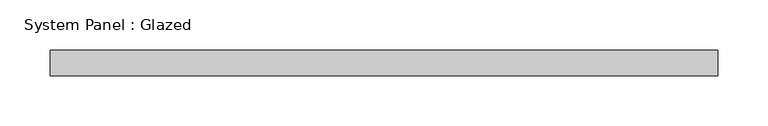
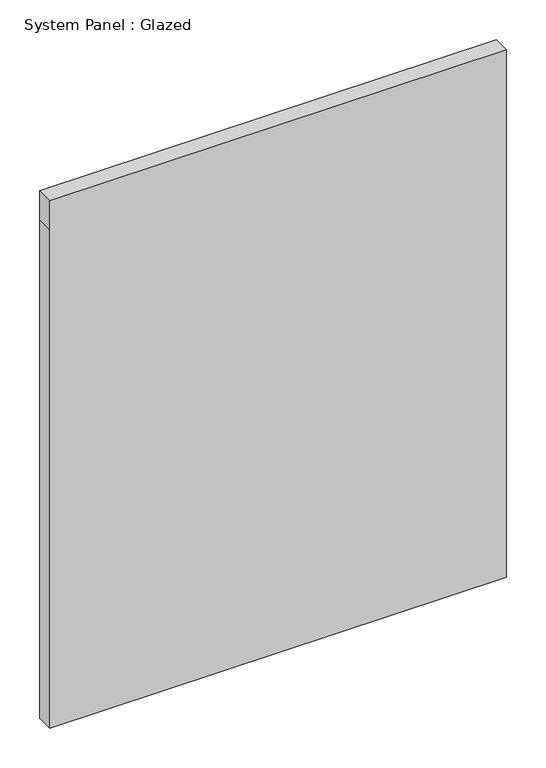
"""IFC4 building model written with IfcOpenShell, lengths in millimetres: plate geometry, System Panel : Glazed."""

from ifc_helpers import new_model, si_unit, frame, origin, place, context, project, spatial, polyline, outline, extrude, source, transform, mapped, element, save


def system_panel_glazed_21711ca4(model_context):
    return source(origin(), model_context, "Body", "SweptSolid", [
        extrude(outline(polyline([(0.0, -333.375), (0.0, 333.375), (769.0361093, 333.375), (813.4861093, 333.375), (813.4861093, -333.375), (769.0361093, -333.375), (0.0, -333.375)])), frame((0.0, 19.05, 0.0), z_axis=(0.0, 1.0, 0.0), x_axis=(0.0, 0.0, 1.0)), (0.0, 0.0, 1.0), 25.4),
    ])


if __name__ == "__main__":
    model = new_model("IFC4")
    model_context = context("Model", 3, world=origin())
    ifc_project = project(units=[si_unit("LENGTHUNIT", "METRE", prefix="MILLI")], contexts=[model_context])
    site = spatial("IfcSite", under=ifc_project)
    building = spatial("IfcBuilding", under=site)
    placement = place(None, origin())
    system_panel_glazed_shape = system_panel_glazed_21711ca4(model_context)
    element("IfcPlate", 1, ObjectType="System Panel : Glazed", at=placement, inside=building, context=model_context, shape_type="MappedRepresentation", body=[
        mapped(system_panel_glazed_shape, transform((0.0, 0.0, 0.0), x_axis=(1.0, 0.0, 0.0), y_axis=(0.0, 1.0, 0.0), z_axis=(0.0, 0.0, 1.0))),
    ])
    save(model, "model.ifc")

# Revit data of these elements
# Type "System Panel : Glazed"
#   Construction Type Id = "GSP4R"
#   Analytic Construction = "1/8 in Pilkington single glazing"
#   Visual Light Transmittance = 0.9
#   Solar Heat Gain Coefficient = 0.86
#   Heat Transfer Coefficient (U) = 1.18115 BTU/(h·ft²·°F)
#   Define Thermal Properties by = 1
# Element 1 (IfcPlate, "System Panel : Glazed")
#   Materials on its faces: "Glass"
# Materials
#   "Glass": class "Glass", colour RGB 0 128 192, transparency 0.75, Description = "Soda Lime Glass", Cost = 0
